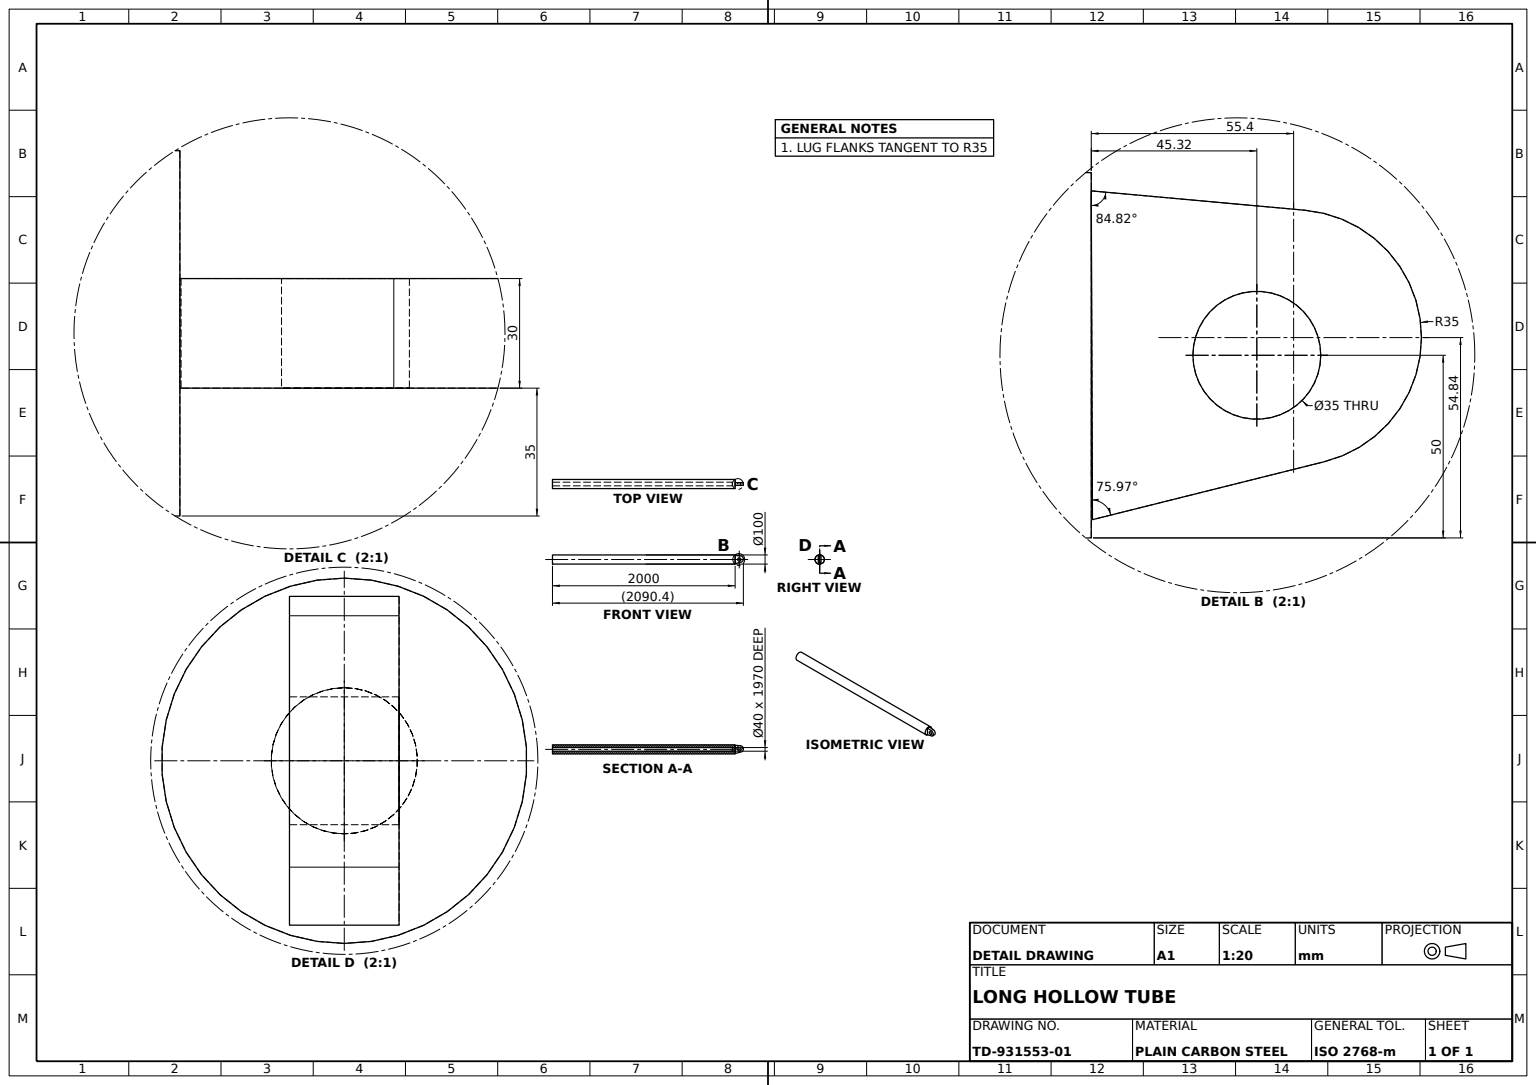
SolidWorks part; units mm, degrees
material "Plain Carbon Steel"
ref_plane "Front Plane" through (0, 0, 0) normal (0, 0, 1) x (1, 0, 0)
ref_plane "Top Plane" through (0, 0, 0) normal (0, 1, 0) x (1, 0, 0)
ref_plane "Right Plane" through (0, 0, 0) normal (1, 0, 0) x (0, 0, -1)
sketch "Tube Profile Ø100" plane through (0, 0, 0) normal (0, 0, 1) x (1, 0, 0)
  circle A0 centre (0, 0) radius 50
  dimension "D1" = 100
extrude "Tube Ø100x2000" add sketch "Tube Profile Ø100" along normal blind 2000
shell "Tube Shell 30 Wall" thickness 30
sketch "Eye Lug Profile" plane through (0, 0, 0) normal (0, 1, 0) x (1, 0, 0)
  line L0 (-45, 0) -> (-39.6959, 58.555)
  line L1 (29.1174, 63.8822) -> (44.9988, 0.3243)
  line L2 (-45, 0) -> (44.9988, 0.3243)
  line L3 (50, 0) -> (-50, 0) construction
  circle A0 centre (0, 45.3243) radius 17.5
  arc A1 (-39.6959, 58.555) -> (29.1174, 63.8822) centre (-4.8386, 55.3975) cw
  dimension "D1" = 35
  dimension "D2" = 35
  dimension "D3" = 45
  dimension "D4" = 45
  dimension "D5" = 45
  dimension "D6" = 5.3041
  dimension "D7" = 40.1614
  dimension "D8" = 74.1174
extrude "Eye Lug 30 Thick" add sketch "Eye Lug Profile" along normal mid plane 30 separate body
